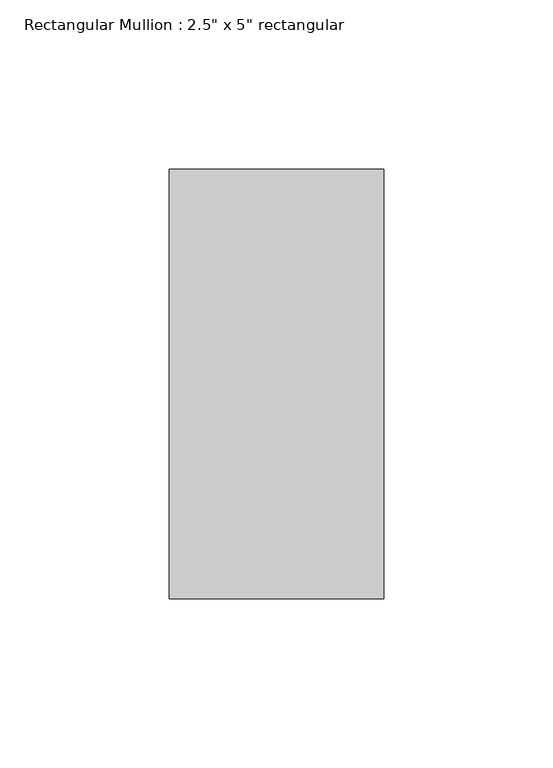
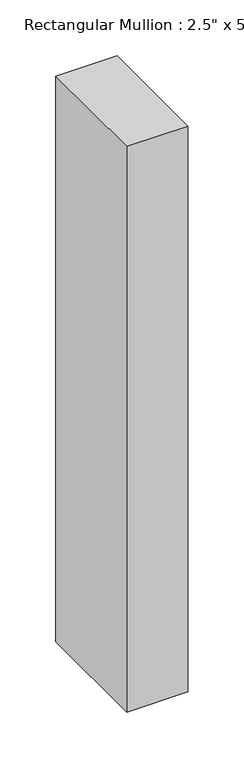
"""IFC4 building model written with IfcOpenShell, lengths in millimetres: member geometry."""

from ifc_helpers import new_model, si_unit, frame, origin, place, context, project, spatial, polyline, outline, extrude, source, transform, mapped, element, save


def member_d8a11517(model_context):
    return source(origin(), model_context, "Body", "SweptSolid", [
        extrude(outline(polyline([(0.0, 63.5), (0.0, -63.5), (-63.5, -63.5), (-63.5, 63.5), (0.0, 63.5)])), frame((0.0, 0.0, -619.76), z_axis=(0.0, 0.0, 1.0), x_axis=(1.0, 0.0, 0.0)), (0.0, 0.0, 1.0), 619.76),
    ])


if __name__ == "__main__":
    model = new_model("IFC4")
    model_context = context("Model", 3, world=origin())
    ifc_project = project(units=[si_unit("LENGTHUNIT", "METRE", prefix="MILLI")], contexts=[model_context])
    site = spatial("IfcSite", under=ifc_project)
    building = spatial("IfcBuilding", under=site)
    placement = place(None, origin())
    member_shape = member_d8a11517(model_context)
    element("IfcMember", 1, ObjectType="Rectangular Mullion : 2.5\" x 5\" rectangular", at=placement, inside=building, context=model_context, shape_type="MappedRepresentation", body=[
        mapped(member_shape, transform((0.0, 0.0, 0.0), x_axis=(1.0, 0.0, 0.0), y_axis=(0.0, 1.0, 0.0), z_axis=(0.0, 0.0, 1.0))),
    ])
    save(model, "model.ifc")

# Revit data of these elements
# Type "Rectangular Mullion : 2.5\" x 5\" rectangular"
#   built-in parameter 1007304 = 0.416667 (stored number, unit not read)
#   built-in parameter 1007301 = 0.104167 (stored number, unit not read)
#   built-in parameter 1007300 = 0.104167 (stored number, unit not read)
# Element 1 (IfcMember, "Rectangular Mullion : 2.5\" x 5\" rectangular")
#   Materials on its faces: "Aluminum"
# Materials
#   "Aluminum": class "Metal", colour RGB 247 247 247, transparency 0, Description = "Aluminum 6061", Cost = 0
